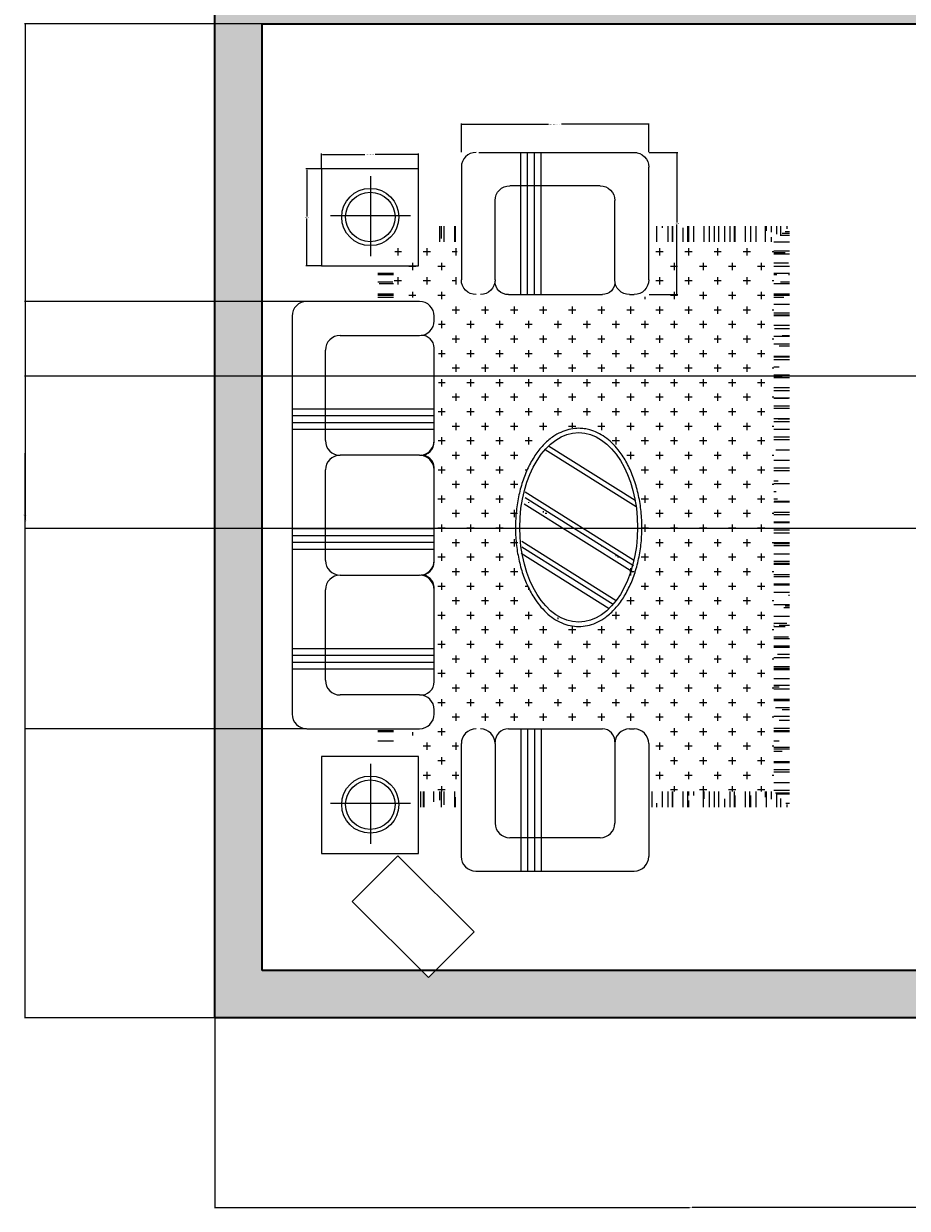
# Model space of a CAD drawing. Units: inches. Extents: x -29 to 404, y -32 to 761.
# Tile 1 of 5: x -29 to 139, y -32 to 193. Entities that reach past the tile are written whole.
import ezdxf

# ---------------------------------------------------------------- set-up
doc = ezdxf.new("R2010")
doc.units = ezdxf.units.IN
doc.header["$MEASUREMENT"] = 0
for name, color, linetype, lineweight in [('A-ANNO-DIMS', 2, 'Continuous', 18), ('A-FLOR-PATT', 9, 'Continuous', 13), ('A-FURN', 8, 'Continuous', 18), ('A-WALL', 7, 'Continuous', 35)]:
    doc.layers.add(name, color=color, linetype=linetype, lineweight=lineweight)
doc.layers.add('A-WALL-PATT', color=251, linetype='Continuous', lineweight=13, true_color=0x636466)
doc.styles.get("Standard").update_dxf_attribs({"font": 'arial.ttf'})
doc.dimstyles.get("Standard").update_dxf_attribs({"dimtxt": 0.18, "dimasz": 0.18, "dimexe": 0.18, "dimexo": 0.0625, "dimgap": 0.09, "dimtad": 0, "dimtih": 1, "dimtoh": 1, "dimdec": 4, "dimzin": 0, "dimdsep": 46, "dimtxsty": 'Standard', "dimcen": 0.09, "dimadec": 0, "dimazin": 0, "dimtfac": 1, "dimtdec": 4, "dimtofl": 0, "dimtmove": 0, "dimatfit": 3, "dimfxl": 1, "dimtolj": 1, "dimtzin": 0, "dimarcsym": 0})

# ---------------------------------------------------------------- blocks, each defined once
blk = doc.blocks.new('END-TABLE-DRAWING')
for p, q in [((9.36, 1.83), (9.36, 17.03)), ((16.95, 9.53), (1.74, 9.53))]:
    blk.add_line(p, q)
blk.add_lwpolyline([(0, 18.43), (0, 0), (18.43, 0), (18.43, 18.43)], close=True)
for radius in [5.44, 4.7]:
    blk.add_circle((9.28, 9.29), radius)
blk = doc.blocks.new('ARMCHAIR-DRAWING')
for p, q in [((8.95, 27.02), (26.84, 27.02)), ((11.3, 26.96), (11.3, 0)), ((12.6, 26.96), (12.6, 0)), ((13.9, 26.96), (13.9, 0)), ((15.2, 26.96), (15.2, 0)), ((31.97, 27.02), (32.86, 27.02)), ((0, 2.79), (0, 24.23)), ((6.41, 24.23), (6.41, 9.13)), ((29.2, 24.48), (29.19, 9.13)), ((35.65, 24.23), (35.65, 2.79)), ((26.4, 6.34), (9.2, 6.34))]:
    blk.add_line(p, q)
for centre, radius, start, end in [((2.79, 24.23), 2.79, 90, 180), ((3.62, 24.23), 2.79, 0, 90), ((8.92, 24.51), 2.51, 89.3411, 180.6299), ((26.84, 24.67), 2.35, 357.014, 90), ((31.97, 24.23), 2.79, 90, 180), ((32.86, 24.23), 2.79, 0, 90), ((9.2, 9.13), 2.79, 180, 270), ((26.4, 9.13), 2.79, 270, 0), ((32.86, 2.79), 2.79, 270, 0)]:
    blk.add_arc(centre, radius, start, end)
blk = doc.blocks.new('*D19')
at = {"layer": 'A-ANNO-DIMS', "color": 0, "lineweight": -2, "transparency": 16777216}
for p, q in [((27.96, 165.88), (27.96, 168.76)), ((28.14, 168.58), (36.21, 168.58)), ((46.21, 168.58), (38.14, 168.58)), ((46.39, 165.88), (46.39, 168.76))]:
    blk.add_line(p, q, dxfattribs=at)
at = {"layer": 'A-ANNO-DIMS', "color": 0, "transparency": 16777216}
for points in [[(28.14, 168.61), (28.14, 168.55), (27.96, 168.58)], [(46.21, 168.61), (46.21, 168.55), (46.39, 168.58)]]:
    blk.add_solid(points, dxfattribs=at)
at = {"layer": 'Defpoints', "color": 0, "transparency": 16777216}
for p in [(46.39, 168.58), (27.96, 165.82), (46.39, 165.82)]:
    blk.add_point(p, dxfattribs=at)
at = {"layer": 'A-ANNO-DIMS', "color": 0, "transparency": 16777216, "insert": (37.17, 168.58), "char_height": 0.18, "attachment_point": 5}
blk.add_mtext('\\A1;TABLE 18 TYP.', dxfattribs=at)
blk = doc.blocks.new('*D20')
at = {"layer": 'A-ANNO-DIMS', "color": 0, "lineweight": -2, "transparency": 16777216}
for p, q in [((27.9, 165.82), (25.01, 165.82)), ((25.19, 165.64), (25.19, 156.78)), ((25.19, 147.57), (25.19, 156.42)), ((27.9, 147.39), (25.01, 147.39))]:
    blk.add_line(p, q, dxfattribs=at)
at = {"layer": 'A-ANNO-DIMS', "color": 0, "transparency": 16777216}
for points in [[(25.16, 165.64), (25.22, 165.64), (25.19, 165.82)], [(25.16, 147.57), (25.22, 147.57), (25.19, 147.39)]]:
    blk.add_solid(points, dxfattribs=at)
at = {"layer": 'Defpoints', "color": 0, "transparency": 16777216}
for p in [(25.19, 165.82), (27.96, 165.82), (27.96, 147.39)]:
    blk.add_point(p, dxfattribs=at)
at = {"layer": 'A-ANNO-DIMS', "color": 0, "transparency": 16777216, "insert": (25.19, 156.6), "char_height": 0.18, "attachment_point": 5}
blk.add_mtext('\\A1;18 TYP.', dxfattribs=at)
blk = doc.blocks.new('*D23')
at = {"layer": 'A-ANNO-DIMS', "color": 0, "lineweight": -2, "transparency": 16777216}
for p, q in [((54.56, 169.01), (54.56, 174.48)), ((54.74, 174.3), (71.14, 174.3)), ((90.03, 174.3), (73.62, 174.3)), ((90.21, 169.01), (90.21, 174.48))]:
    blk.add_line(p, q, dxfattribs=at)
at = {"layer": 'A-ANNO-DIMS', "color": 0, "transparency": 16777216}
for points in [[(54.74, 174.33), (54.74, 174.27), (54.56, 174.3)], [(90.03, 174.33), (90.03, 174.27), (90.21, 174.3)]]:
    blk.add_solid(points, dxfattribs=at)
at = {"layer": 'Defpoints', "color": 0, "transparency": 16777216}
for p in [(90.21, 174.3), (54.56, 168.95), (90.21, 168.95)]:
    blk.add_point(p, dxfattribs=at)
at = {"layer": 'A-ANNO-DIMS', "color": 0, "transparency": 16777216, "insert": (72.38, 174.3), "char_height": 0.18, "attachment_point": 5}
blk.add_mtext('\\A1;ARMCHAIR 36 TYP.', dxfattribs=at)
blk = doc.blocks.new('*D24')
at = {"layer": 'A-ANNO-DIMS', "color": 0, "lineweight": -2, "transparency": 16777216}
for p, q in [((90.27, 168.95), (95.74, 168.95)), ((95.56, 168.77), (95.56, 155.62)), ((95.56, 142.1), (95.56, 155.26)), ((90.27, 141.92), (95.74, 141.92))]:
    blk.add_line(p, q, dxfattribs=at)
at = {"layer": 'A-ANNO-DIMS', "color": 0, "transparency": 16777216}
for points in [[(95.53, 168.77), (95.59, 168.77), (95.56, 168.95)], [(95.53, 142.1), (95.59, 142.1), (95.56, 141.92)]]:
    blk.add_solid(points, dxfattribs=at)
at = {"layer": 'Defpoints', "color": 0, "transparency": 16777216}
for p in [(90.21, 168.95), (90.21, 141.92), (95.56, 141.92)]:
    blk.add_point(p, dxfattribs=at)
at = {"layer": 'A-ANNO-DIMS', "color": 0, "transparency": 16777216, "insert": (95.56, 155.44), "char_height": 0.18, "attachment_point": 5}
blk.add_mtext('\\A1;27 TYP.', dxfattribs=at)
blk = doc.blocks.new('*D33')
at = {"layer": 'A-ANNO-DIMS', "color": 0, "lineweight": -2, "transparency": 16777216}
for p, q in [((16.62, 193.43), (-28.55, 193.43)), ((-28.37, 193.25), (-28.37, 99.12)), ((-28.37, 4.61), (-28.37, 98.75)), ((7.62, 4.43), (-28.55, 4.43))]:
    blk.add_line(p, q, dxfattribs=at)
at = {"layer": 'A-ANNO-DIMS', "color": 0, "transparency": 16777216}
for points in [[(-28.4, 193.25), (-28.34, 193.25), (-28.37, 193.43)], [(-28.4, 4.61), (-28.34, 4.61), (-28.37, 4.43)]]:
    blk.add_solid(points, dxfattribs=at)
at = {"layer": 'Defpoints', "color": 0, "transparency": 16777216}
for p in [(-28.37, 193.43), (16.68, 193.43), (7.68, 4.43)]:
    blk.add_point(p, dxfattribs=at)
at = {"layer": 'A-ANNO-DIMS', "color": 0, "transparency": 16777216, "insert": (-28.37, 98.93), "char_height": 0.18, "attachment_point": 5}
blk.add_mtext('\\A1;189', dxfattribs=at)
blk = doc.blocks.new('*D38')
at = {"layer": 'A-ANNO-DIMS', "color": 0, "lineweight": -2, "transparency": 16777216}
for p, q in [((7.68, 4.37), (7.68, -31.8)), ((188.68, 4.37), (188.68, -31.8)), ((7.86, -31.62), (97.92, -31.62)), ((188.5, -31.62), (98.44, -31.62))]:
    blk.add_line(p, q, dxfattribs=at)
at = {"layer": 'A-ANNO-DIMS', "color": 0, "transparency": 16777216}
for points in [[(7.86, -31.59), (7.86, -31.65), (7.68, -31.62)], [(188.5, -31.59), (188.5, -31.65), (188.68, -31.62)]]:
    blk.add_solid(points, dxfattribs=at)
at = {"layer": 'Defpoints', "color": 0, "transparency": 16777216}
for p in [(7.68, 4.43), (188.68, 4.43), (188.68, -31.62)]:
    blk.add_point(p, dxfattribs=at)
at = {"layer": 'A-ANNO-DIMS', "color": 0, "transparency": 16777216, "insert": (98.18, -31.62), "char_height": 0.18, "attachment_point": 5}
blk.add_mtext('\\A1;181', dxfattribs=at)
blk = doc.blocks.new('*D46')
at = {"layer": 'A-ANNO-DIMS', "color": 0, "lineweight": -2, "transparency": 16777216}
for p, q in [((238.62, 126.43), (-28.55, 126.43)), ((-28.37, 126.25), (-28.37, 112.12)), ((-28.37, 97.61), (-28.37, 111.75)), ((238.62, 97.43), (-28.55, 97.43))]:
    blk.add_line(p, q, dxfattribs=at)
at = {"layer": 'A-ANNO-DIMS', "color": 0, "transparency": 16777216}
for points in [[(-28.4, 126.25), (-28.34, 126.25), (-28.37, 126.43)], [(-28.4, 97.61), (-28.34, 97.61), (-28.37, 97.43)]]:
    blk.add_solid(points, dxfattribs=at)
at = {"layer": 'Defpoints', "color": 0, "transparency": 16777216}
for p in [(-28.37, 126.43), (238.68, 126.43), (238.68, 97.43)]:
    blk.add_point(p, dxfattribs=at)
at = {"layer": 'A-ANNO-DIMS', "color": 0, "transparency": 16777216, "insert": (-28.37, 111.93), "char_height": 0.18, "attachment_point": 5}
blk.add_mtext('\\A1;29', dxfattribs=at)
blk = doc.blocks.new('*D58')
at = {"layer": 'A-ANNO-DIMS', "color": 0, "lineweight": -2, "transparency": 16777216}
for p, q in [((25.1, 140.62), (-28.55, 140.62)), ((-28.37, 140.44), (-28.37, 100.19)), ((-28.37, 59.57), (-28.37, 99.83)), ((25.1, 59.39), (-28.55, 59.39))]:
    blk.add_line(p, q, dxfattribs=at)
at = {"layer": 'A-ANNO-DIMS', "color": 0, "transparency": 16777216}
for points in [[(-28.4, 140.44), (-28.34, 140.44), (-28.37, 140.62)], [(-28.4, 59.57), (-28.34, 59.57), (-28.37, 59.39)]]:
    blk.add_solid(points, dxfattribs=at)
at = {"layer": 'Defpoints', "color": 0, "transparency": 16777216}
for p in [(-28.37, 140.62), (25.16, 140.62), (25.16, 59.39)]:
    blk.add_point(p, dxfattribs=at)
at = {"layer": 'A-ANNO-DIMS', "color": 0, "transparency": 16777216, "insert": (-28.37, 100.01), "char_height": 0.18, "attachment_point": 5}
blk.add_mtext('\\A1;81.23', dxfattribs=at)

msp = doc.modelspace()

# ---------------------------------------------------------------- hatches: boundary and pattern name
at = {"layer": 'A-FLOR-PATT'}
h = msp.add_hatch(dxfattribs=at)
h.set_pattern_fill('AR-RROOF', color=256, scale=3.276796, angle=270, style=0)
h.set_pattern_definition([(180, (365.949, 512.927), (-6.488057, 2.949117), [44.23675, -5.89823, 14.74558, -2.94912]), (180, (362.0267, 514.4014), (2.949117, 3.922325), [8.84735, -0.97321, 17.6947, -2.21184]), (180, (364.4745, 515.4336), (-15.335407, 1.975908), [23.592934, -4.12876, 11.79647, -2.94912])])
h.paths.add_polyline_path([(38.683, 56.802), (38.683, 59.392), (41.632, 59.392), (41.632, 56.802)])
h.paths.add_polyline_path([(113.993, 47.435), (113.993, 151.958), (116.942, 154.907), (116.942, 44.486)])
h.paths.add_polyline_path([(38.683, 140.624), (38.683, 147.466), (41.632, 147.079), (41.632, 140.624)])
h = msp.add_hatch(dxfattribs=at)
h.set_pattern_fill('AR-RROOF', color=256, scale=3.276796, angle=180, style=0)
h.set_pattern_definition([(270, (365.949, 512.927), (-2.949117, -6.488057), [44.23675, -5.89823, 14.74558, -2.94912]), (270, (364.4745, 509.0045), (-3.922325, 2.949117), [8.84735, -0.97321, 17.6947, -2.21184]), (270, (363.4423, 511.4523), (-1.975908, -15.335407), [23.592934, -4.12876, 11.79647, -2.94912])])
h.paths.add_polyline_path([(46.39, 44.486), (46.39, 47.435), (54.558, 47.435), (54.558, 44.486)])
h.paths.add_polyline_path([(90.209, 44.486), (90.209, 47.435), (113.993, 47.435), (116.942, 44.486)])
h.paths.add_polyline_path([(90.209, 151.958), (90.209, 154.907), (116.942, 154.907), (113.993, 151.958)])
h.paths.add_polyline_path([(49.964, 151.958), (50.351, 154.907), (54.558, 154.907), (54.558, 151.958)])
h = msp.add_hatch(dxfattribs=at)
h.set_pattern_fill('CROSS', color=256, scale=12.287986, angle=180, style=0)
h.set_pattern_definition([(270, (365.949, 512.9269), (-2.764797, -2.764797), [1.382398, -4.147195]), (180, (366.6402, 512.2357), (-2.764797, 2.764797), [1.382398, -4.147195])])
h.paths.add_polyline_path([(91.117, 47.435), (90.82, 57.773), (90.643, 59.9), (56.099, 60.077), (53.973, 58.836), (54.096, 47.435), (46.39, 47.435), (46.39, 56.802), (41.632, 56.802), (41.632, 58.619), (49.899, 58.836), (50.253, 139.485), (49.013, 141.435), (41.632, 141.332), (41.632, 148.345), (42.154, 151.958), (53.814, 151.958), (53.619, 143.385), (56.099, 141.08), (85.86, 140.549), (90.643, 141.789), (90.971, 151.958), (113.993, 151.958), (113.993, 47.435)])
h.paths.add_polyline_path([(87.808, 95.173), (87.631, 108.289), (81.608, 115.556), (78.951, 116.62), (75.585, 116.62), (73.105, 116.088), (69.739, 114.493), (68.322, 111.125), (66.374, 107.226), (65.488, 102.972), (64.956, 97.831), (66.905, 87.019), (71.334, 80.815), (78.42, 79.575), (82.494, 81.524), (86.037, 86.665)], flags=16)
edge = h.paths.add_edge_path(flags=0)
edge.add_line((86.23, 90.813), (66.886, 102.445))
edge.add_ellipse((96.794, 97.903), major_axis=(-21.39, 21.39), ratio=1, start_angle=35.87674, end_angle=36.36513, ccw=False)
edge.add_line((66.926, 102.7), (86.288, 91.057))
edge.add_ellipse((56.823, 97.903), major_axis=(21.39, 21.39), ratio=1, start_angle=301.44538, end_angle=301.92024, ccw=False)
edge.add_line((86.23, 90.813), (86.23, 90.813))
edge.add_ellipse((66.694, 95.525), major_axis=(14.21, 14.21), ratio=0.9999999, start_angle=301.43989, end_angle=301.45625)
edge.add_line((86.232, 90.819), (86.232, 90.819))
edge.add_line((86.232, 90.819), (86.232, 90.819))
edge.add_line((86.232, 90.819), (86.232, 90.819))
edge.add_line((86.232, 90.819), (86.232, 90.819))
edge.add_line((86.232, 90.819), (86.232, 90.819))
edge.add_ellipse((66.694, 95.525), major_axis=(-14.21, 14.21), ratio=1, start_angle=211.43989, end_angle=211.45624, ccw=False)
at = {"layer": 'A-WALL-PATT'}
h = msp.add_hatch(color=256, dxfattribs=at)
h.dxf.hatch_style = 1
h.paths.add_polyline_path([(188.678, 415.434), (183.678, 415.434), (183.678, 287.434), (180.678, 287.434), (180.678, 282.434), (183.678, 282.434), (183.678, 198.434), (57.678, 198.434), (57.678, 282.434), (144.678, 282.434), (144.678, 287.434), (16.678, 287.434), (16.678, 548.434), (144.678, 548.434, -0.1168354), (148.504, 564.585), (148.451, 564.616), (149.501, 566.434), (180.678, 548.434), (180.678, 543.434), (183.678, 543.434), (191.678, 543.434), (191.678, 548.434), (191.678, 553.634), (225.453, 573.134), (226.591, 571.164), (226.533, 571.131, -0.1168354), (230.678, 553.634), (230.678, 548.434), (358.678, 548.434), (358.678, 471.434), (322.678, 471.434), (322.678, 543.434), (358.678, 543.434), (358.678, 548.434), (230.678, 548.434), (230.678, 543.434), (233.678, 543.434), (252.678, 543.434), (252.678, 466.434), (260.678, 466.434), (260.678, 471.434), (257.678, 471.434), (257.678, 543.434), (317.678, 543.434), (317.678, 471.434), (296.678, 471.434), (296.678, 466.434), (358.678, 466.434), (358.678, 198.434), (286.678, 198.434), (286.678, 193.434), (358.678, 193.434), (358.678, 97.434), (238.678, 97.434), (238.678, 193.434), (250.678, 193.434), (250.678, 198.434), (233.678, 198.434), (233.678, 92.434), (358.678, 92.434), (358.678, 13.434), (296.678, 13.434), (296.678, 4.434), (367.678, 4.434), (367.678, 724.434), (7.678, 724.434), (7.678, 4.434), (188.678, 4.434), (188.678, 13.434), (188.678, 154.434), (183.678, 154.434), (183.678, 13.434), (49.651, 13.434), (48.286, 12.069), (46.92, 13.434), (16.678, 13.434), (16.678, 193.434), (183.678, 193.434), (183.678, 190.434), (188.678, 190.434)])
h.paths.add_polyline_path([(52.678, 282.434), (52.678, 198.434), (16.678, 198.434), (16.678, 282.434)], flags=16)

# ---------------------------------------------------------------- linework, layer by layer
at = {"layer": 'A-FURN'}
for p, q in [((87.966, 168.871), (57.887, 168.871)), ((46.594, 140.624), (25.159, 140.624)), ((22.367, 137.832), (22.367, 62.184)), ((49.386, 136.944), (49.386, 137.967)), ((31.502, 134.152), (46.594, 134.152)), ((28.71, 114.163), (28.71, 131.36)), ((49.386, 113.909), (49.386, 131.804)), ((49.323, 120.159), (22.367, 120.159)), ((49.323, 118.858), (22.367, 118.858)), ((49.323, 117.557), (22.367, 117.557)), ((49.323, 116.257), (22.367, 116.257)), ((71.147, 113.156), (87.603, 102.835)), ((46.594, 111.371), (31.502, 111.371)), ((70.498, 112.486), (87.799, 101.634)), ((28.71, 91.382), (28.71, 108.579)), ((49.386, 91.128), (49.386, 109.023)), ((66.685, 104.444), (87.298, 91.515)), ((66.531, 102.135), (87.144, 89.206)), ((66.685, 103.366), (87.298, 90.437)), ((49.323, 97.378), (22.367, 97.378)), ((49.323, 96.077), (22.367, 96.077)), ((49.323, 94.777), (22.367, 94.777)), ((66.07, 95.055), (84.02, 83.796)), ((49.323, 93.476), (22.367, 93.476)), ((65.916, 92.746), (82.661, 82.243)), ((66.07, 93.977), (83.445, 83.079)), ((31.502, 88.582), (46.594, 88.582)), ((28.71, 68.593), (28.71, 85.79)), ((49.386, 68.339), (49.386, 86.234)), ((49.323, 74.589), (22.367, 74.589)), ((49.323, 73.288), (22.367, 73.288)), ((49.323, 71.988), (22.367, 71.988)), ((49.323, 70.687), (22.367, 70.687)), ((46.594, 65.801), (31.502, 65.801)), ((49.386, 62.184), (49.386, 63.009)), ((25.159, 59.392), (46.594, 59.392)), ((57.287, 32.324), (87.365, 32.324))]:
    msp.add_line(p, q, dxfattribs=at)
msp.add_lwpolyline([(33.804, 26.55), (42.493, 35.239), (56.974, 20.758), (48.286, 12.069)], close=True, dxfattribs=at)
for centre, radius, start, end in [((57.35, 166.157), 2.792, 90, 180), ((25.159, 137.832), 2.792, 90, 180), ((46.594, 137.832), 2.792, 0, 90), ((46.594, 136.944), 2.792, 270, 0), ((31.502, 131.36), 2.792, 90, 180), ((47.035, 131.804), 2.351, 0, 92.98595), ((31.502, 114.163), 2.792, 180, 270), ((46.594, 114.163), 2.792, 270, 0), ((46.877, 113.88), 2.51, 269.37008, 0.65888), ((31.502, 108.579), 2.792, 90, 180), ((46.594, 108.579), 2.792, 0, 90), ((47.035, 109.023), 2.351, 0, 92.98595), ((31.502, 91.382), 2.792, 180, 270), ((46.594, 91.374), 2.792, 270, 0), ((46.877, 91.099), 2.51, 269.37008, 0.65888), ((31.502, 85.79), 2.792, 90, 180), ((46.594, 85.798), 2.792, 0, 90), ((47.035, 86.234), 2.351, 0, 92.98595), ((31.502, 68.593), 2.792, 180, 270), ((46.854, 68.32), 2.532, 264.10185, 0.44553), ((46.594, 63.009), 2.792, 0, 90), ((25.159, 62.184), 2.792, 180, 270), ((46.594, 62.184), 2.792, 270, 0), ((57.298, 35.116), 2.792, 180, 270)]:
    msp.add_arc(centre, radius, start, end, dxfattribs=at)
at = {"layer": 'A-FURN', "extrusion": (0, 0, -1)}
msp.add_ellipse((76.87, 97.667), major_axis=(0, 18.017), ratio=0.6218602, start_param=4.712389, end_param=10.9955743, dxfattribs=at)
at = {"layer": 'A-FURN'}
msp.add_open_spline([(76.87, 116.503), (77.226, 116.503), (77.583, 116.479), (78.291, 116.381), (78.643, 116.308), (79.49, 116.073), (79.981, 115.887), (80.939, 115.423), (81.406, 115.145), (82.31, 114.505), (82.746, 114.143), (83.584, 113.341), (83.986, 112.902), (84.902, 111.761), (85.398, 111.025), (86.301, 109.437), (86.709, 108.585), (87.424, 106.787), (87.733, 105.842), (88.246, 103.884), (88.449, 102.872), (88.746, 100.809), (88.839, 99.758), (88.912, 97.646), (88.893, 96.585), (88.741, 94.484), (88.609, 93.443), (88.237, 91.41), (87.996, 90.418), (87.411, 88.51), (87.068, 87.594), (86.285, 85.864), (85.846, 85.049), (84.882, 83.545), (84.357, 82.855), (83.234, 81.621), (82.635, 81.077), (81.522, 80.26), (81.021, 79.954), (79.989, 79.448), (79.46, 79.247), (78.383, 78.959), (77.837, 78.872), (76.739, 78.813), (76.189, 78.841), (75.098, 79.014), (74.559, 79.158), (73.502, 79.556), (72.985, 79.809), (71.983, 80.418), (71.498, 80.773), (70.568, 81.577), (70.123, 82.025), (69.276, 83.005), (68.876, 83.538), (68.021, 84.834), (67.582, 85.621), (66.796, 87.296), (66.448, 88.183), (65.85, 90.034), (65.6, 90.998), (65.204, 92.975), (65.058, 93.99), (64.873, 96.042), (64.835, 97.08), (64.866, 99.152), (64.936, 100.186), (65.182, 102.222), (65.358, 103.224), (65.814, 105.171), (66.093, 106.115), (66.747, 107.919), (67.122, 108.78), (67.96, 110.395), (68.423, 111.15), (69.427, 112.531), (69.969, 113.158), (71.118, 114.266), (71.727, 114.747), (72.837, 115.443), (73.327, 115.696), (74.329, 116.101), (74.841, 116.254), (75.859, 116.454), (76.365, 116.503), (76.87, 116.503)], degree=3, knots=[3.1415927, 3.1415927, 3.1415927, 3.1415927, 3.2269172, 3.2269172, 3.3122416, 3.3122416, 3.4342667, 3.4342667, 3.5562918, 3.5562918, 3.6783168, 3.6783168, 3.8003419, 3.8003419, 3.9715738, 3.9715738, 4.1428058, 4.1428058, 4.3140377, 4.3140377, 4.4852697, 4.4852697, 4.6565016, 4.6565016, 4.8277335, 4.8277335, 4.9989655, 4.9989655, 5.1701974, 5.1701974, 5.3414293, 5.3414293, 5.5126613, 5.5126613, 5.6838932, 5.6838932, 5.8551252, 5.8551252, 5.9866911, 5.9866911, 6.118257, 6.118257, 6.2498229, 6.2498229, 6.3813888, 6.3813888, 6.5129547, 6.5129547, 6.6445207, 6.6445207, 6.7760866, 6.7760866, 6.9076525, 6.9076525, 7.0392184, 7.0392184, 7.2070156, 7.2070156, 7.3748129, 7.3748129, 7.5426101, 7.5426101, 7.7104073, 7.7104073, 7.8782046, 7.8782046, 8.0460018, 8.0460018, 8.213799, 8.213799, 8.3815962, 8.3815962, 8.5493935, 8.5493935, 8.7171907, 8.7171907, 8.8849879, 8.8849879, 9.0527852, 9.0527852, 9.178207, 9.178207, 9.3036288, 9.3036288, 9.424778, 9.424778, 9.424778, 9.424778], dxfattribs=at)
at = {"layer": 'A-WALL'}
for p, q in [((16.678, 193.434), (183.678, 193.434)), ((16.678, 13.434), (16.678, 193.434)), ((183.678, 13.434), (16.678, 13.434))]:
    msp.add_line(p, q, dxfattribs=at)
msp.add_lwpolyline([(188.678, 4.434), (7.678, 4.434), (7.678, 724.434), (367.678, 724.434), (367.678, 4.434), (296.678, 4.434)], dxfattribs=at)

# ---------------------------------------------------------------- block references
at = {"layer": 'A-FURN', "extrusion": (0, 0, -1), "zscale": -1, "rotation": 180}
msp.add_blockref('ARMCHAIR-DRAWING', (-54.558, 168.949), dxfattribs=at)
at = {"layer": 'A-FURN'}
for name, p in [('END-TABLE-DRAWING', (27.958, 147.386)), ('ARMCHAIR-DRAWING', (54.558, 32.324)), ('END-TABLE-DRAWING', (27.958, 35.665))]:
    msp.add_blockref(name, p, dxfattribs=at)

# ---------------------------------------------------------------- dimensions: what is measured, and where the dimension line sits
at = {"layer": 'A-ANNO-DIMS'}
for base, p1, p2, override, picture, middle in [((-28.372, 193.434), (7.678, 4.434), (16.678, 193.434), {"dimdec": 0, "dimlfac": 1, "dimrnd": 0, "dimzin": 0, "dimdsep": 46, "dimlunit": 2}, '*D33', (-28.372, 98.934)), ((-28.372, 140.624), (25.159, 59.392), (25.159, 140.624), {"dimdec": 2, "dimlfac": 1, "dimrnd": 0, "dimzin": 0, "dimdsep": 46, "dimlunit": 2}, '*D58', (-28.372, 100.008)), ((-28.372, 126.434), (238.678, 97.434), (238.678, 126.434), {"dimdec": 0, "dimlfac": 1, "dimrnd": 0, "dimzin": 0, "dimdsep": 46, "dimlunit": 2}, '*D46', (-28.372, 111.934))]:
    dim = msp.add_linear_dim(base=base, p1=p1, p2=p2, angle=90, dimstyle='Standard', override=override, dxfattribs=at)
    dim.commit()
    dim.dimension.update_dxf_attribs({"geometry": picture, "text_midpoint": middle})
for base, p1, p2, text, picture, middle in [((90.209, 174.297), (54.558, 168.949), (90.209, 168.949), 'ARMCHAIR <> TYP.', '*D23', (72.384, 174.297)), ((46.39, 168.583), (27.958, 165.818), (46.39, 165.818), 'TABLE <> TYP.', '*D19', (37.174, 168.583))]:
    dim = msp.add_linear_dim(base=base, p1=p1, p2=p2, text=text, dimstyle='Standard', override={"dimdec": 0, "dimlfac": 1, "dimrnd": 0, "dimzin": 0, "dimdsep": 46, "dimlunit": 2}, dxfattribs=at)
    dim.commit()
    dim.dimension.update_dxf_attribs({"geometry": picture, "text_midpoint": middle})
for base, p1, p2, angle, picture, middle in [((95.557, 141.922), (90.209, 168.949), (90.209, 141.922), 270, '*D24', (95.557, 155.436)), ((25.193, 165.818), (27.958, 147.386), (27.958, 165.818), 90, '*D20', (25.193, 156.602))]:
    dim = msp.add_linear_dim(base=base, p1=p1, p2=p2, angle=angle, text='<> TYP.', dimstyle='Standard', override={"dimdec": 0, "dimlfac": 1, "dimrnd": 0, "dimzin": 0, "dimdsep": 46, "dimlunit": 2}, dxfattribs=at)
    dim.commit()
    dim.dimension.update_dxf_attribs({"geometry": picture, "text_midpoint": middle})
dim = msp.add_linear_dim(base=(188.678, -31.616), p1=(7.678, 4.434), p2=(188.678, 4.434), dimstyle='Standard', override={"dimdec": 0, "dimlfac": 1, "dimrnd": 0, "dimzin": 0, "dimdsep": 46, "dimlunit": 2}, dxfattribs=at)
dim.commit()
dim.dimension.update_dxf_attribs({"geometry": '*D38', "text_midpoint": (98.178, -31.616)})

doc.saveas('drawing.dxf')
